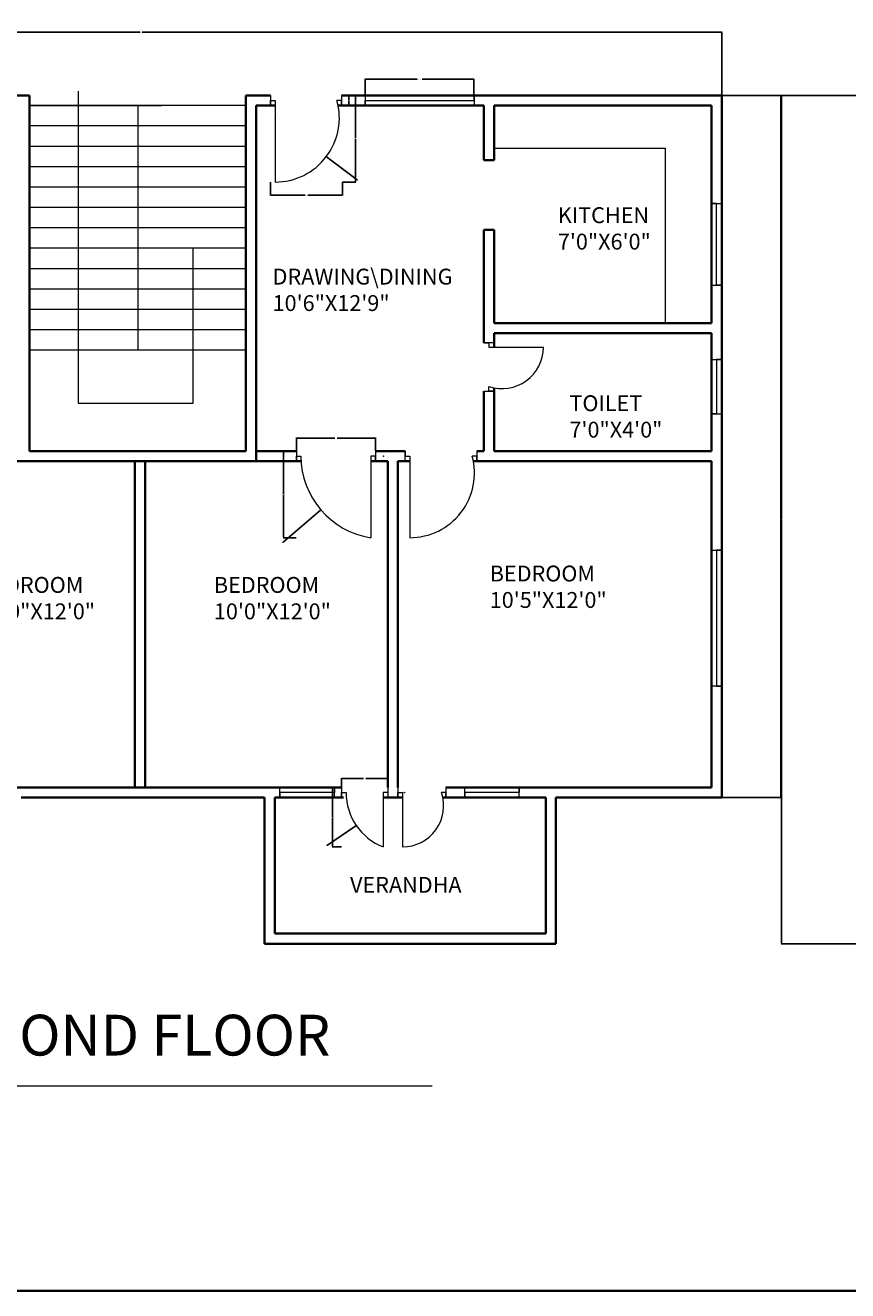
# Model space of a CAD drawing. Units: inches. Extents: x 2055 to 3558, y 1520 to 2888.
# Tile 2 of 8: x 2369 to 2732, y 1520 to 2079. Entities that reach past the tile are written whole.
import ezdxf

# ---------------------------------------------------------------- set-up
doc = ezdxf.new("R2010")
doc.units = ezdxf.units.IN
for name, color, linetype, lineweight in [('A-ANNO-DIMS', 2, 'Continuous', 18), ('A-ANNO-TEXT', 7, 'Continuous', 18), ('A-ANNO-TTLB', 7, 'Continuous', 35), ('A-AREA-IDEN', 7, 'Continuous', 18), ('A-DOOR', 3, 'Continuous', 18), ('A-FLOR-FIXT', 8, 'Continuous', 18), ('A-FLOR-STRS', 7, 'Continuous', 18), ('A-GLAZ', 4, 'Continuous', 18), ('A-WALL', 7, 'Continuous', 35)]:
    doc.layers.add(name, color=color, linetype=linetype, lineweight=lineweight)
doc.styles.get("Standard").update_dxf_attribs({"font": 'arial.ttf'})
doc.dimstyles.get("Standard").update_dxf_attribs({"dimtxt": 0.18, "dimasz": 0.18, "dimexe": 0.18, "dimexo": 0.0625, "dimgap": 0.09, "dimtad": 0, "dimtih": 1, "dimtoh": 1, "dimdec": 4, "dimzin": 0, "dimdsep": 46, "dimtxsty": 'Standard', "dimcen": 0.09, "dimadec": 0, "dimazin": 0, "dimtfac": 1, "dimtdec": 4, "dimtofl": 0, "dimtmove": 0, "dimatfit": 3, "dimfxl": 1, "dimtolj": 1, "dimtzin": 0, "dimarcsym": 0})

# ---------------------------------------------------------------- blocks, each defined once
blk = doc.blocks.new('DOOR-BATH-24-B')
for p, q in [((4.5, 21.32), (0, 21.32)), ((0, 21.32), (2.25, 21.32)), ((2.25, 21.32), (2.25, 19.32)), ((2.25, 19.32), (26.25, 19.32)), ((0, 0), (4.5, 0)), ((2.25, 0), (2.25, 2)), ((4.5, 0), (2.25, 0))]:
    blk.add_line(p, q)
blk.add_arc((8, 19.32), 18.25, 251.6403, 0)
blk = doc.blocks.new('DOOR-ENTRY-36-D')
for p, q in [((0, 38.25), (0, 33.75)), ((0, 33.75), (0, 36)), ((0, 36), (2, 36)), ((2, 36), (2, 0)), ((31.26, 36), (29.26, 36)), ((31.26, 38.25), (31.26, 33.75)), ((31.26, 33.75), (31.26, 36))]:
    blk.add_line(p, q)
blk.add_arc((2, 28.32), 28.32, 270, 15.7411)
blk = doc.blocks.new('DOOR-BED-36-F')
for p, q in [((0, 33.75), (0, 38.25)), ((0, 38.25), (0, 36)), ((0, 36), (2, 36)), ((2, 36), (2, 0)), ((31.57, 36), (29.57, 36)), ((31.57, 38.25), (31.57, 33.75)), ((31.57, 33.75), (31.57, 36))]:
    blk.add_line(p, q)
blk.add_arc((2, 28.56), 28.56, 270, 15.1117)
blk = doc.blocks.new('DOOR-BED-36-G')
for p, q in [((0, 38.25), (0, 33.75)), ((0, 33.75), (0, 36)), ((0, 36), (2, 36)), ((34.89, 36), (32.89, 36)), ((32.89, 36), (32.89, 0)), ((34.89, 38.25), (34.89, 33.75)), ((34.89, 33.75), (34.89, 36))]:
    blk.add_line(p, q)
blk.add_arc((38.42, 36), 36.42, 180, 261.253)
blk = doc.blocks.new('DOOR-VERANDA-24-A')
for p, q in [((0, 26.25), (0, 21.75)), ((0, 21.75), (0, 24)), ((0, 24), (2, 24)), ((2, 24), (2, 0)), ((21.18, 24), (19.18, 24)), ((21.18, 26.25), (21.18, 21.75)), ((21.18, 21.75), (21.18, 24))]:
    blk.add_line(p, q)
blk.add_arc((2, 18.15), 18.15, 270, 18.8194)
blk = doc.blocks.new('DOOR-VERANDA-24-B')
for p, q in [((0, 26.25), (0, 21.75)), ((0, 21.75), (0, 24)), ((0, 24), (2, 24)), ((20.42, 24), (18.42, 24)), ((18.42, 24), (18.42, 0)), ((20.42, 26.25), (20.42, 21.75))]:
    blk.add_line(p, q)
blk.add_arc((27.75, 24), 25.75, 180, 248.7547)
blk = doc.blocks.new('WIN-36')
for p, q in [((2.25, 36), (0, 36)), ((0, 36), (4.5, 36)), ((2.25, 0), (2.25, 36)), ((0, 0), (4.5, 0)), ((4.5, 0), (2.25, 0))]:
    blk.add_line(p, q)
blk = doc.blocks.new('WIN-24')
for p, q in [((0, 24), (4.5, 24)), ((4.5, 24), (2.25, 24)), ((2.25, 24), (2.25, 0)), ((2.25, 0), (0, 0)), ((0, 0), (4.5, 0))]:
    blk.add_line(p, q)
blk = doc.blocks.new('WIN-60-2')
for p, q in [((4.5, 60), (0, 60)), ((0, 60), (2.25, 60)), ((2.25, 60), (2.25, 0)), ((2.25, 0), (0, 0)), ((0, 0), (4.5, 0))]:
    blk.add_line(p, q)
blk = doc.blocks.new('WIN-48')
for p, q in [((0, 4.5), (0, 0)), ((0, 0), (0, 2.25)), ((0, 2.25), (48, 2.25)), ((48, 2.25), (48, 4.5)), ((48, 4.5), (48, 0))]:
    blk.add_line(p, q)
blk = doc.blocks.new('COUNTER-4')
for p, q in [((0, 77.26), (75.5, 77.26)), ((75.5, 77.26), (75.5, 0))]:
    blk.add_line(p, q)
blk = doc.blocks.new('VERANDA-PERIMETER')
for p, q in [((0, 0), (0, 64.5)), ((4.5, 64.5), (4.5, 4.5)), ((124.15, 4.5), (124.15, 64.5)), ((128.65, 64.5), (128.65, 4.5)), ((4.5, 0), (0, 0)), ((4.5, 4.5), (124.15, 4.5)), ((128.65, 0), (4.5, 0)), ((128.65, 4.5), (128.65, 0))]:
    blk.add_line(p, q)
blk = doc.blocks.new('STAIR-RETURN')
for p, q in [((21.46, 137.78), (21.46, 0)), ((95.44, 131.38), (0, 131.38)), ((0, 131.38), (58.19, 131.38)), ((47.72, 131.38), (47.72, 23.38)), ((95.44, 122.38), (0, 122.38)), ((95.44, 113.38), (0, 113.38)), ((95.44, 104.38), (0, 104.38)), ((95.44, 95.38), (0, 95.38)), ((95.44, 86.38), (0, 86.38)), ((95.44, 77.38), (0, 77.38)), ((95.44, 68.38), (0, 68.38)), ((72.2, 0), (72.2, 68.38)), ((95.44, 59.38), (0, 59.38)), ((95.44, 50.38), (0, 50.38)), ((95.44, 41.38), (0, 41.38)), ((95.44, 32.38), (0, 32.38)), ((95.44, 23.38), (0, 23.38)), ((21.46, 0), (72.2, 0))]:
    blk.add_line(p, q)
blk = doc.blocks.new('*D72')
at = {"layer": 'A-ANNO-DIMS', "color": 0, "lineweight": -2, "transparency": 16777216}
for p, q in [((2509.29, 2048), (2515.15, 2048)), ((2514.97, 2047.82), (2514.97, 2029.06)), ((2514.97, 2009.93), (2514.97, 2028.69)), ((2509.29, 2009.75), (2515.15, 2009.75))]:
    blk.add_line(p, q, dxfattribs=at)
at = {"layer": 'A-ANNO-DIMS', "color": 0, "transparency": 16777216}
for points in [[(2514.94, 2047.82), (2515, 2047.82), (2514.97, 2048)], [(2514.94, 2009.93), (2515, 2009.93), (2514.97, 2009.75)]]:
    blk.add_solid(points, dxfattribs=at)
at = {"layer": 'Defpoints', "color": 0, "transparency": 16777216}
for p in [(2509.23, 2048), (2514.97, 2048), (2509.23, 2009.75)]:
    blk.add_point(p, dxfattribs=at)
at = {"layer": 'A-ANNO-DIMS', "color": 0, "transparency": 16777216, "insert": (2514.97, 2028.87), "char_height": 0.18, "attachment_point": 5}
blk.add_mtext('\\A1;ENTRY DOOR 38 TYP.', dxfattribs=at)
blk = doc.blocks.new('*D73')
at = {"layer": 'A-ANNO-DIMS', "color": 0, "lineweight": -2, "transparency": 16777216}
for p, q in [((2477.57, 2009.69), (2477.57, 2003.83)), ((2509.23, 2009.69), (2509.23, 2003.83)), ((2477.75, 2004.01), (2492.87, 2004.01)), ((2509.05, 2004.01), (2493.93, 2004.01))]:
    blk.add_line(p, q, dxfattribs=at)
at = {"layer": 'A-ANNO-DIMS', "color": 0, "transparency": 16777216}
for points in [[(2477.75, 2004.04), (2477.75, 2003.98), (2477.57, 2004.01)], [(2509.05, 2004.04), (2509.05, 2003.98), (2509.23, 2004.01)]]:
    blk.add_solid(points, dxfattribs=at)
at = {"layer": 'Defpoints', "color": 0, "transparency": 16777216}
for p in [(2477.57, 2009.75), (2509.23, 2009.75), (2509.23, 2004.01)]:
    blk.add_point(p, dxfattribs=at)
at = {"layer": 'A-ANNO-DIMS', "color": 0, "transparency": 16777216, "insert": (2493.4, 2004.01), "char_height": 0.18, "attachment_point": 5}
blk.add_mtext('\\A1;32 TYP.', dxfattribs=at)
blk = doc.blocks.new('*D80')
at = {"layer": 'A-ANNO-DIMS', "color": 0, "lineweight": -2, "transparency": 16777216}
for p, q in [((2488.87, 1891), (2483.02, 1891)), ((2483.2, 1890.82), (2483.2, 1872.06)), ((2483.2, 1852.93), (2483.2, 1871.69)), ((2488.87, 1852.75), (2483.02, 1852.75))]:
    blk.add_line(p, q, dxfattribs=at)
at = {"layer": 'A-ANNO-DIMS', "color": 0, "transparency": 16777216}
for points in [[(2483.17, 1890.82), (2483.23, 1890.82), (2483.2, 1891)], [(2483.17, 1852.93), (2483.23, 1852.93), (2483.2, 1852.75)]]:
    blk.add_solid(points, dxfattribs=at)
at = {"layer": 'Defpoints', "color": 0, "transparency": 16777216}
for p in [(2483.2, 1891), (2488.93, 1891), (2488.93, 1852.75)]:
    blk.add_point(p, dxfattribs=at)
at = {"layer": 'A-ANNO-DIMS', "color": 0, "transparency": 16777216, "insert": (2483.2, 1871.87), "char_height": 0.18, "attachment_point": 5}
blk.add_mtext('\\A1;BED DOOR 38 TYP.', dxfattribs=at)
blk = doc.blocks.new('*D81')
at = {"layer": 'A-ANNO-DIMS', "color": 0, "lineweight": -2, "transparency": 16777216}
for p, q in [((2488.93, 1891.06), (2488.93, 1896.92)), ((2489.11, 1896.74), (2505.85, 1896.74)), ((2523.64, 1896.74), (2506.9, 1896.74)), ((2523.82, 1891.06), (2523.82, 1896.92))]:
    blk.add_line(p, q, dxfattribs=at)
at = {"layer": 'A-ANNO-DIMS', "color": 0, "transparency": 16777216}
for points in [[(2489.11, 1896.77), (2489.11, 1896.71), (2488.93, 1896.74)], [(2523.64, 1896.77), (2523.64, 1896.71), (2523.82, 1896.74)]]:
    blk.add_solid(points, dxfattribs=at)
at = {"layer": 'Defpoints', "color": 0, "transparency": 16777216}
for p in [(2523.82, 1896.74), (2488.93, 1891), (2523.82, 1891)]:
    blk.add_point(p, dxfattribs=at)
at = {"layer": 'A-ANNO-DIMS', "color": 0, "transparency": 16777216, "insert": (2506.38, 1896.74), "char_height": 0.18, "attachment_point": 5}
blk.add_mtext('\\A1;35 TYP.', dxfattribs=at)
blk = doc.blocks.new('*D84')
at = {"layer": 'A-ANNO-DIMS', "color": 0, "lineweight": -2, "transparency": 16777216}
for p, q in [((2508.79, 1742.5), (2504.74, 1742.5)), ((2504.92, 1742.32), (2504.92, 1729.56)), ((2504.92, 1716.43), (2504.92, 1729.19)), ((2508.79, 1716.25), (2504.74, 1716.25))]:
    blk.add_line(p, q, dxfattribs=at)
at = {"layer": 'A-ANNO-DIMS', "color": 0, "transparency": 16777216}
for points in [[(2504.89, 1742.32), (2504.95, 1742.32), (2504.92, 1742.5)], [(2504.89, 1716.43), (2504.95, 1716.43), (2504.92, 1716.25)]]:
    blk.add_solid(points, dxfattribs=at)
at = {"layer": 'Defpoints', "color": 0, "transparency": 16777216}
for p in [(2504.92, 1742.5), (2508.85, 1742.5), (2508.85, 1716.25)]:
    blk.add_point(p, dxfattribs=at)
at = {"layer": 'A-ANNO-DIMS', "color": 0, "transparency": 16777216, "insert": (2504.92, 1729.37), "char_height": 0.18, "attachment_point": 5}
blk.add_mtext('\\A1;VERANDA DOOR 26 TYP.', dxfattribs=at)
blk = doc.blocks.new('*D85')
at = {"layer": 'A-ANNO-DIMS', "color": 0, "lineweight": -2, "transparency": 16777216}
for p, q in [((2508.85, 1742.56), (2508.85, 1746.62)), ((2509.03, 1746.44), (2518.53, 1746.44)), ((2529.09, 1746.44), (2519.59, 1746.44)), ((2529.27, 1742.56), (2529.27, 1746.62))]:
    blk.add_line(p, q, dxfattribs=at)
at = {"layer": 'A-ANNO-DIMS', "color": 0, "transparency": 16777216}
for points in [[(2509.03, 1746.47), (2509.03, 1746.41), (2508.85, 1746.44)], [(2529.09, 1746.47), (2529.09, 1746.41), (2529.27, 1746.44)]]:
    blk.add_solid(points, dxfattribs=at)
at = {"layer": 'Defpoints', "color": 0, "transparency": 16777216}
for p in [(2529.27, 1746.44), (2508.85, 1742.5), (2529.27, 1742.5)]:
    blk.add_point(p, dxfattribs=at)
at = {"layer": 'A-ANNO-DIMS', "color": 0, "transparency": 16777216, "insert": (2519.06, 1746.44), "char_height": 0.18, "attachment_point": 5}
blk.add_mtext('\\A1;20 TYP.', dxfattribs=at)
blk = doc.blocks.new('*D102')
at = {"layer": 'A-ANNO-DIMS', "color": 0, "lineweight": -2, "transparency": 16777216}
for p, q in [((2519.32, 2048.06), (2519.32, 2055.38)), ((2519.5, 2055.2), (2542.2, 2055.2)), ((2567.14, 2055.2), (2544.44, 2055.2)), ((2567.32, 2048.06), (2567.32, 2055.38))]:
    blk.add_line(p, q, dxfattribs=at)
at = {"layer": 'A-ANNO-DIMS', "color": 0, "transparency": 16777216}
for points in [[(2519.5, 2055.23), (2519.5, 2055.17), (2519.32, 2055.2)], [(2567.14, 2055.23), (2567.14, 2055.17), (2567.32, 2055.2)]]:
    blk.add_solid(points, dxfattribs=at)
at = {"layer": 'Defpoints', "color": 0, "transparency": 16777216}
for p in [(2567.32, 2055.2), (2519.32, 2048), (2567.32, 2048)]:
    blk.add_point(p, dxfattribs=at)
at = {"layer": 'A-ANNO-DIMS', "color": 0, "transparency": 16777216, "insert": (2543.32, 2055.2), "char_height": 0.18, "attachment_point": 5}
blk.add_mtext('\\A1;WINDOW 48 TYP.', dxfattribs=at)
blk = doc.blocks.new('*D103')
at = {"layer": 'A-ANNO-DIMS', "color": 0, "lineweight": -2, "transparency": 16777216}
for p, q in [((2519.26, 2048), (2511.94, 2048)), ((2512.12, 2047.82), (2512.12, 2045.93)), ((2512.12, 2043.68), (2512.12, 2045.57)), ((2519.26, 2043.5), (2511.94, 2043.5))]:
    blk.add_line(p, q, dxfattribs=at)
at = {"layer": 'A-ANNO-DIMS', "color": 0, "transparency": 16777216}
for points in [[(2512.09, 2047.82), (2512.15, 2047.82), (2512.12, 2048)], [(2512.09, 2043.68), (2512.15, 2043.68), (2512.12, 2043.5)]]:
    blk.add_solid(points, dxfattribs=at)
at = {"layer": 'Defpoints', "color": 0, "transparency": 16777216}
for p in [(2512.12, 2048), (2519.32, 2048), (2519.32, 2043.5)]:
    blk.add_point(p, dxfattribs=at)
at = {"layer": 'A-ANNO-DIMS', "color": 0, "transparency": 16777216, "insert": (2512.12, 2045.75), "char_height": 0.18, "attachment_point": 5}
blk.add_mtext('\\A1;5 TYP.', dxfattribs=at)
blk = doc.blocks.new('*D121')
at = {"layer": 'A-ANNO-DIMS', "color": 0, "lineweight": -2, "transparency": 16777216}
for p, q in [((2164.17, 2048.06), (2164.17, 2076.13)), ((2164.35, 2075.95), (2420.03, 2075.95)), ((2676.49, 2075.95), (2420.82, 2075.95)), ((2676.67, 2048.06), (2676.67, 2076.13))]:
    blk.add_line(p, q, dxfattribs=at)
at = {"layer": 'A-ANNO-DIMS', "color": 0, "transparency": 16777216}
for points in [[(2164.35, 2075.98), (2164.35, 2075.92), (2164.17, 2075.95)], [(2676.49, 2075.98), (2676.49, 2075.92), (2676.67, 2075.95)]]:
    blk.add_solid(points, dxfattribs=at)
at = {"layer": 'Defpoints', "color": 0, "transparency": 16777216}
for p in [(2676.67, 2075.95), (2164.17, 2048), (2676.67, 2048)]:
    blk.add_point(p, dxfattribs=at)
at = {"layer": 'A-ANNO-DIMS', "color": 0, "transparency": 16777216, "insert": (2420.42, 2075.95), "char_height": 0.18, "attachment_point": 5}
blk.add_mtext('\\A1;512.5', dxfattribs=at)
blk = doc.blocks.new('*D123')
at = {"layer": 'A-ANNO-DIMS', "color": 0, "lineweight": -2, "transparency": 16777216}
for p, q in [((2676.74, 2048), (2702.9, 2048)), ((2702.72, 2047.82), (2702.72, 1893.18)), ((2702.72, 1738.18), (2702.72, 1892.82)), ((2676.74, 1738), (2702.9, 1738))]:
    blk.add_line(p, q, dxfattribs=at)
at = {"layer": 'A-ANNO-DIMS', "color": 0, "transparency": 16777216}
for points in [[(2702.69, 2047.82), (2702.75, 2047.82), (2702.72, 2048)], [(2702.69, 1738.18), (2702.75, 1738.18), (2702.72, 1738)]]:
    blk.add_solid(points, dxfattribs=at)
at = {"layer": 'Defpoints', "color": 0, "transparency": 16777216}
for p in [(2676.67, 2048), (2676.67, 1738), (2702.72, 1738)]:
    blk.add_point(p, dxfattribs=at)
at = {"layer": 'A-ANNO-DIMS', "color": 0, "transparency": 16777216, "insert": (2702.72, 1893), "char_height": 0.18, "attachment_point": 5}
blk.add_mtext('\\A1;310', dxfattribs=at)
blk = doc.blocks.new('*D134')
at = {"layer": 'A-ANNO-DIMS', "color": 0, "lineweight": -2, "transparency": 16777216}
for p, q in [((2791.43, 2048), (2702.83, 2048)), ((2703.01, 2047.82), (2703.01, 1860.93)), ((2703.01, 1673.68), (2703.01, 1860.57)), ((2866, 1673.5), (2702.83, 1673.5))]:
    blk.add_line(p, q, dxfattribs=at)
at = {"layer": 'A-ANNO-DIMS', "color": 0, "transparency": 16777216}
for points in [[(2702.98, 2047.82), (2703.04, 2047.82), (2703.01, 2048)], [(2702.98, 1673.68), (2703.04, 1673.68), (2703.01, 1673.5)]]:
    blk.add_solid(points, dxfattribs=at)
at = {"layer": 'Defpoints', "color": 0, "transparency": 16777216}
for p in [(2791.5, 2048), (2703.01, 1673.5), (2866.07, 1673.5)]:
    blk.add_point(p, dxfattribs=at)
at = {"layer": 'A-ANNO-DIMS', "color": 0, "transparency": 16777216, "insert": (2703.01, 1860.75), "char_height": 0.18, "attachment_point": 5}
blk.add_mtext('\\A1;374.5', dxfattribs=at)
blk = doc.blocks.new('*D175')
at = {"layer": 'A-ANNO-DIMS', "color": 0, "lineweight": -2, "transparency": 16777216}
for p, q in [((2527.27, 1888.75), (2527.45, 1888.75)), ((2527.36, 1888.66), (2527.36, 1888.84)), ((2483.13, 1850.8), (2499.58, 1864.92)), ((2482.95, 1850.8), (2483.13, 1850.8))]:
    blk.add_line(p, q, dxfattribs=at)
at = {"layer": 'A-ANNO-DIMS', "color": 0, "transparency": 16777216}
blk.add_solid([(2499.56, 1864.94), (2499.6, 1864.89), (2499.71, 1865.03)], dxfattribs=at)
at = {"layer": 'Defpoints', "color": 0, "transparency": 16777216}
for p in [(2527.36, 1888.75), (2499.71, 1865.03)]:
    blk.add_point(p, dxfattribs=at)
at = {"layer": 'A-ANNO-DIMS', "color": 0, "transparency": 16777216, "insert": (2482.47, 1850.8), "char_height": 0.18, "attachment_point": 5}
blk.add_mtext('\\A1;R36.42', dxfattribs=at)
blk = doc.blocks.new('*D178')
at = {"layer": 'A-ANNO-DIMS', "color": 0, "lineweight": -2, "transparency": 16777216}
for p, q in [((2479.48, 2038.07), (2479.66, 2038.07)), ((2479.57, 2037.98), (2479.57, 2038.16)), ((2515.69, 2010.72), (2502.29, 2020.87)), ((2515.87, 2010.72), (2515.69, 2010.72))]:
    blk.add_line(p, q, dxfattribs=at)
at = {"layer": 'A-ANNO-DIMS', "color": 0, "transparency": 16777216}
blk.add_solid([(2502.3, 2020.89), (2502.27, 2020.84), (2502.14, 2020.97)], dxfattribs=at)
at = {"layer": 'Defpoints', "color": 0, "transparency": 16777216}
for p in [(2479.57, 2038.07), (2502.14, 2020.97)]:
    blk.add_point(p, dxfattribs=at)
at = {"layer": 'A-ANNO-DIMS', "color": 0, "transparency": 16777216, "insert": (2516.35, 2010.72), "char_height": 0.18, "attachment_point": 5}
blk.add_mtext('\\A1;R28.32', dxfattribs=at)
blk = doc.blocks.new('*D179')
at = {"layer": 'A-ANNO-DIMS', "color": 0, "lineweight": -2, "transparency": 16777216}
for p, q in [((2536.51, 1740.25), (2536.69, 1740.25)), ((2536.6, 1740.16), (2536.6, 1740.34)), ((2502.6, 1716.99), (2515.2, 1725.61)), ((2502.42, 1716.99), (2502.6, 1716.99))]:
    blk.add_line(p, q, dxfattribs=at)
at = {"layer": 'A-ANNO-DIMS', "color": 0, "transparency": 16777216}
blk.add_solid([(2515.19, 1725.63), (2515.22, 1725.58), (2515.35, 1725.71)], dxfattribs=at)
at = {"layer": 'Defpoints', "color": 0, "transparency": 16777216}
for p in [(2536.6, 1740.25), (2515.35, 1725.71)]:
    blk.add_point(p, dxfattribs=at)
at = {"layer": 'A-ANNO-DIMS', "color": 0, "transparency": 16777216, "insert": (2501.94, 1716.99), "char_height": 0.18, "attachment_point": 5}
blk.add_mtext('\\A1;R25.75', dxfattribs=at)

msp = doc.modelspace()

# ---------------------------------------------------------------- linework, layer by layer
at = {"layer": 'A-ANNO-TEXT'}
msp.add_line((2201.7713, 1610.7234), (2548.8845, 1610.7234), dxfattribs=at)
at = {"layer": 'A-ANNO-TTLB'}
msp.add_lwpolyline([(2054.7598, 2888.2545), (3557.8479, 2888.2545), (3557.8479, 1520.3256), (2054.7598, 1520.3256)], close=True, dxfattribs=at)
at = {"layer": 'A-WALL'}
for p, q in [((2360.2558, 2047.9995), (2371.1747, 2047.9995)), ((2371.1747, 2043.4995), (2371.1747, 2047.9995)), ((2466.6196, 2047.9995), (2477.5665, 2047.9995)), ((2466.6196, 2043.4995), (2466.6196, 2047.9995)), ((2466.6196, 2047.9995), (2477.5665, 2047.9995)), ((2508.8221, 2047.9995), (2676.6747, 2047.9995)), ((2676.6747, 2047.9995), (2676.6747, 1737.9995)), ((2371.1747, 2043.4995), (2371.1747, 1890.9995)), ((2466.6196, 2043.4995), (2466.6196, 1890.9995)), ((2471.1196, 2043.4995), (2471.1196, 1947.4995)), ((2471.1196, 2043.4995), (2471.1196, 1886.4995)), ((2479.5665, 2043.4995), (2471.1196, 2043.4995)), ((2571.6747, 2043.4995), (2507.3582, 2043.4995)), ((2571.6747, 2043.4995), (2571.6747, 2019.4149)), ((2576.1747, 2043.4995), (2576.1747, 2019.4149)), ((2576.1747, 2043.4995), (2672.1747, 2043.4995)), ((2672.1747, 2043.4995), (2672.1747, 1947.4995)), ((2571.6747, 2019.4149), (2576.1747, 2019.4149)), ((2571.6747, 1988.6064), (2576.1747, 1988.6064)), ((2571.6747, 1988.6064), (2571.6747, 1938.8165)), ((2576.1747, 1988.6064), (2576.1747, 1947.4995)), ((2576.1747, 1947.4995), (2672.1747, 1947.4995)), ((2576.1747, 1942.9995), (2672.1747, 1942.9995)), ((2576.1747, 1942.9995), (2576.1747, 1936.8165)), ((2672.1747, 1942.9995), (2672.1747, 1890.9995)), ((2571.6747, 1917.4944), (2571.6747, 1890.9995)), ((2576.1747, 1918.9038), (2576.1747, 1890.9995)), ((2371.1747, 1890.9995), (2422.6747, 1890.9995)), ((2422.6747, 1890.9995), (2466.6196, 1890.9995)), ((2450.1747, 1890.9995), (2466.6196, 1890.9995)), ((2471.1196, 1890.9995), (2488.9334, 1890.9995)), ((2523.8181, 1890.9995), (2536.9825, 1890.9995)), ((2568.5506, 1890.9995), (2571.6747, 1890.9995)), ((2576.1747, 1890.9995), (2672.1747, 1890.9995)), ((2337.3301, 1886.4995), (2422.6747, 1886.4995)), ((2417.6747, 1886.4995), (2417.6747, 1742.4995)), ((2422.1747, 1886.4995), (2422.1747, 1742.4995)), ((2422.6747, 1886.4995), (2491.003, 1886.4995)), ((2521.8181, 1886.4995), (2529.2739, 1886.4995)), ((2529.2739, 1886.4995), (2529.2739, 1742.4995)), ((2533.7739, 1886.4995), (2533.7739, 1742.4995)), ((2533.7739, 1886.4995), (2538.9825, 1886.4995)), ((2567.0616, 1886.4995), (2672.1747, 1886.4995)), ((2576.1747, 1886.4995), (2672.1747, 1886.4995)), ((2672.1747, 1886.4995), (2672.1747, 1742.4995)), ((2323.5061, 1742.4995), (2508.8547, 1742.4995)), ((2367.3911, 1737.9995), (2422.6747, 1737.9995)), ((2371.1747, 1742.4995), (2445.6747, 1742.4995)), ((2422.6747, 1742.4995), (2445.6747, 1742.4995)), ((2422.6747, 1737.9995), (2474.8449, 1737.9995)), ((2450.1747, 1742.4995), (2508.8547, 1742.4995)), ((2479.3449, 1737.9995), (2509.6541, 1737.9995)), ((2527.2739, 1737.9995), (2535.7739, 1737.9995)), ((2553.5587, 1737.9995), (2598.991, 1737.9995)), ((2554.9501, 1742.4995), (2672.1747, 1742.4995)), ((2554.9501, 1742.4995), (2571.6747, 1742.4995)), ((2576.1747, 1742.4995), (2672.1747, 1742.4995)), ((2603.491, 1737.9995), (2676.6747, 1737.9995))]:
    msp.add_line(p, q, dxfattribs=at)

# ---------------------------------------------------------------- block references
at = {"layer": 'A-DOOR'}
for name, p in [('DOOR-ENTRY-36-D', (2477.566, 2009.749)), ('DOOR-BATH-24-B', (2571.675, 1917.494)), ('DOOR-BED-36-G', (2488.933, 1852.749)), ('DOOR-BED-36-F', (2536.983, 1852.749)), ('DOOR-VERANDA-24-B', (2508.855, 1716.249)), ('DOOR-VERANDA-24-A', (2533.774, 1716.249))]:
    msp.add_blockref(name, p, dxfattribs=at)
at = {"layer": 'A-FLOR-FIXT'}
msp.add_blockref('COUNTER-4', (2576.175, 1947.499), dxfattribs=at)
at = {"layer": 'A-FLOR-STRS'}
msp.add_blockref('STAIR-RETURN', (2371.175, 1912.12), dxfattribs=at)
at = {"layer": 'A-GLAZ'}
for name, p in [('WIN-48', (2519.323, 2043.499)), ('WIN-36', (2672.175, 1964.2795)), ('WIN-24', (2672.175, 1907.4213))]:
    msp.add_blockref(name, p, dxfattribs=at)
at = {"layer": 'A-GLAZ', "extrusion": (0, 0, -1), "zscale": -1}
msp.add_blockref('WIN-60-2', (-2676.6743, 1787.2273), dxfattribs=at)
at = {"layer": 'A-GLAZ', "extrusion": (0, 0, -1), "zscale": -1, "rotation": 90}
for p in [(-2481.6854, 1737.9998), (-2563.312, 1737.9998)]:
    msp.add_blockref('WIN-24', p, dxfattribs=at)
at = {"layer": 'A-WALL'}
msp.add_blockref('VERANDA-PERIMETER', (2474.8449, 1673.499), dxfattribs=at)

# ---------------------------------------------------------------- texts
at = {"layer": 'A-ANNO-TEXT', "insert": (2211.3331, 1642.1482), "char_height": 18, "attachment_point": 1}
msp.add_mtext_dynamic_manual_height_columns('FIRST OR SECOND FLOOR ', width=532.043788, gutter_width=12.5, heights=[0], dxfattribs=at)
at = {"layer": 'A-AREA-IDEN', "char_height": 7, "attachment_point": 1}
for s, width, insert in [('KITCHEN\\P7\'0"X6\'0"', 92.673757, (2604.3294, 1998.6234)), ('DRAWING\\\\DINING\\P10\'6"X12\'9"', 76.318653, (2478.4251, 1971.4995)), ('TOILET\\P7\'0"X4\'0"', 58.820839, (2609.4563, 1915.6079)), ('BEDROOM\\P10\'5"X12\'0"', 285.522885, (2574.2596, 1840.4245)), ('BEDROOM\\P10\'0"X12\'0"', 113.389445, (2348.4409, 1835.3994)), ('BEDROOM\\P10\'0"X12\'0"', 113.389445, (2452.5191, 1835.3994)), ('VERANDHA', 73.975505, (2512.6158, 1702.9912))]:
    msp.add_mtext_dynamic_manual_height_columns(s, width=width, gutter_width=12.5, heights=[0], dxfattribs=dict(at, insert=insert))

# ---------------------------------------------------------------- dimensions: what is measured, and where the dimension line sits
at = {"layer": 'A-ANNO-DIMS'}
dim = msp.add_linear_dim(base=(2676.6747, 2075.9495), p1=(2164.1747, 2047.9995), p2=(2676.6747, 2047.9995), dimstyle='Standard', override={"dimdec": 1, "dimlfac": 1, "dimrnd": 0, "dimzin": 0, "dimdsep": 46, "dimlunit": 2}, dxfattribs=at)
dim.commit()
dim.dimension.update_dxf_attribs({"geometry": '*D121', "text_midpoint": (2420.4247, 2075.9495)})
for base, p1, p2, text, picture, middle in [((2567.3225, 2055.1995), (2519.3225, 2047.9995), (2567.3225, 2047.9995), 'WINDOW <> TYP.', '*D102', (2543.3225, 2055.1995)), ((2509.228, 2004.012), (2477.5665, 2009.7495), (2509.228, 2009.7495), '<> TYP.', '*D73', (2493.3972, 2004.012)), ((2523.8181, 1896.737), (2488.9334, 1890.9995), (2523.8181, 1890.9995), '<> TYP.', '*D81', (2506.3758, 1896.737)), ((2529.2739, 1746.437), (2508.8547, 1742.4995), (2529.2739, 1742.4995), '<> TYP.', '*D85', (2519.0643, 1746.437))]:
    dim = msp.add_linear_dim(base=base, p1=p1, p2=p2, text=text, dimstyle='Standard', override={"dimdec": 0, "dimlfac": 1, "dimrnd": 0, "dimzin": 0, "dimdsep": 46, "dimlunit": 2}, dxfattribs=at)
    dim.commit()
    dim.dimension.update_dxf_attribs({"geometry": picture, "text_midpoint": middle})
for base, p1, p2, text, picture, middle in [((2514.9655, 2047.9995), (2509.228, 2009.7495), (2509.228, 2047.9995), 'ENTRY DOOR <> TYP.', '*D72', (2514.9655, 2028.8745)), ((2512.1225164771, 2047.9994988353), (2519.3225164771, 2043.4994988353), (2519.3225164771, 2047.9994988353), '<> TYP.', '*D103', (2512.1225164771, 2045.7494988353)), ((2483.1959, 1890.9995), (2488.9334, 1852.7495), (2488.9334, 1890.9995), 'BED DOOR <> TYP.', '*D80', (2483.1959, 1871.8745)), ((2504.9172, 1742.4995), (2508.8547, 1716.2495), (2508.8547, 1742.4995), 'VERANDA DOOR <> TYP.', '*D84', (2504.9172, 1729.3745))]:
    dim = msp.add_linear_dim(base=base, p1=p1, p2=p2, angle=90, text=text, dimstyle='Standard', override={"dimdec": 0, "dimlfac": 1, "dimrnd": 0, "dimzin": 0, "dimdsep": 46, "dimlunit": 2}, dxfattribs=at)
    dim.commit()
    dim.dimension.update_dxf_attribs({"geometry": picture, "text_midpoint": middle})
for base, p1, p2, override, picture, middle in [((2702.7247, 1737.9995), (2676.6747, 2047.9995), (2676.6747, 1737.9995), {"dimdec": 0, "dimlfac": 1, "dimrnd": 0, "dimzin": 0, "dimdsep": 46, "dimlunit": 2}, '*D123', (2702.7247, 1892.9995)), ((2703.0074, 1673.4995), (2791.4955, 2047.9995), (2866.0658, 1673.4995), {"dimdec": 1, "dimlfac": 1, "dimrnd": 0, "dimzin": 0, "dimdsep": 46, "dimlunit": 2}, '*D134', (2703.0074, 1860.7495))]:
    dim = msp.add_linear_dim(base=base, p1=p1, p2=p2, angle=90, dimstyle='Standard', override=override, dxfattribs=at)
    dim.commit()
    dim.dimension.update_dxf_attribs({"geometry": picture, "text_midpoint": middle})
for center, mpoint, picture, middle in [((2479.5665, 2038.0672), (2502.1432, 2020.9739), '*D178', (2516.3481, 2010.7179)), ((2527.3571, 1888.7495), (2499.7129, 1865.0329), '*D175', (2482.4674, 1850.8029)), ((2536.6047, 1740.2495), (2515.3522, 1725.7101), '*D179', (2501.9401, 1716.9865))]:
    dim = msp.add_radius_dim(center=center, mpoint=mpoint, dimstyle='Standard', override={"dimdec": 2, "dimlfac": 1, "dimrnd": 0, "dimzin": 0, "dimdsep": 46, "dimlunit": 2}, dxfattribs=at)
    dim.commit()
    dim.dimension.update_dxf_attribs({"geometry": picture, "text_midpoint": middle, "dimtype": 164})

doc.saveas('drawing.dxf')
